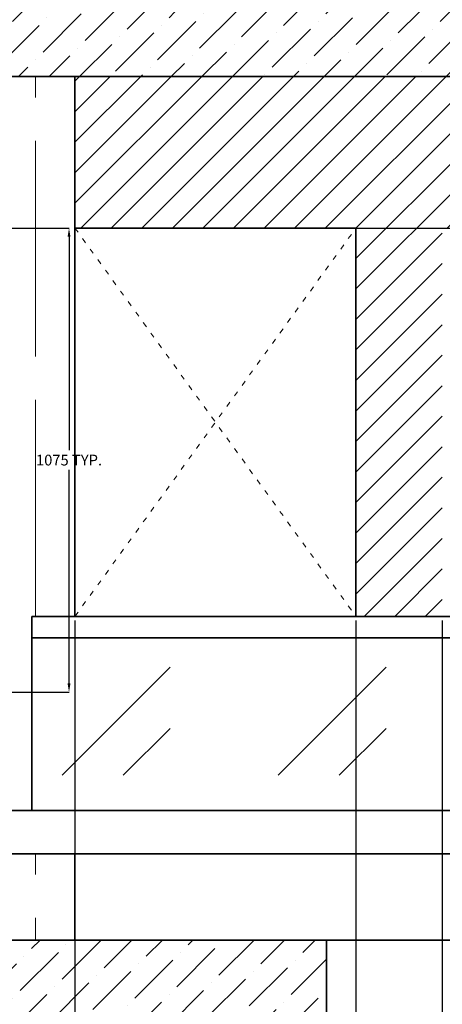
# Model space of a CAD drawing. Units: millimetres. Extents: x -692 to 9639, y -141 to 10345.
# Tile 5 of 19: x 5064 to 6042, y 2699 to 4981. Entities that reach past the tile are written whole.
import ezdxf

# ---------------------------------------------------------------- set-up
doc = ezdxf.new("R2010")
doc.units = ezdxf.units.MM
doc.header["$MEASUREMENT"] = 0
doc.linetypes.add('ACAD_ISO03W100', pattern=[30, 12, -18])
for name, color, linetype, lineweight in [('A-ANNO-DIMS', 2, 'Continuous', 18), ('A-DOOR-SWNG', 3, 'ACAD_ISO03W100', 18), ('A-ELEV', 7, 'Continuous', 35), ('A-ELEV-PATT', 8, 'Continuous', 13)]:
    doc.layers.add(name, color=color, linetype=linetype, lineweight=lineweight)
doc.styles.get("Standard").update_dxf_attribs({"font": 'arial.ttf'})
doc.dimstyles.get("Standard").update_dxf_attribs({"dimtxt": 25, "dimasz": 20, "dimexe": 0.18, "dimexo": 10, "dimgap": 10, "dimtad": 0, "dimtih": 1, "dimtoh": 1, "dimdec": 0, "dimzin": 0, "dimdsep": 46, "dimtxsty": 'Standard', "dimcen": 10, "dimadec": 0, "dimazin": 0, "dimtfac": 1, "dimtdec": 0, "dimtofl": 0, "dimtmove": 0, "dimatfit": 3, "dimfxl": 1, "dimtolj": 1, "dimtzin": 0, "dimarcsym": 0})

# ---------------------------------------------------------------- blocks, each defined once
blk = doc.blocks.new('*D5')
at = {"layer": 'A-ANNO-DIMS', "color": 0, "lineweight": -2, "transparency": 16777216}
for p, q in [((5026.5, 4497.8), (5178, 4497.8)), ((5177.8, 4477.8), (5177.8, 3983)), ((5177.8, 3442.8), (5177.8, 3937.5)), ((5026.5, 3422.8), (5178, 3422.8))]:
    blk.add_line(p, q, dxfattribs=at)
at = {"layer": 'A-ANNO-DIMS', "color": 0, "lineweight": -3, "transparency": 16777216}
for points in [[(5174.5, 4477.8), (5181.1, 4477.8), (5177.8, 4497.8)], [(5174.5, 3442.8), (5181.1, 3442.8), (5177.8, 3422.8)]]:
    blk.add_solid(points, dxfattribs=at)
at = {"layer": 'Defpoints', "color": 0, "lineweight": -3, "transparency": 16777216}
for p in [(5016.5, 4497.8), (5177.8, 4497.8), (5016.5, 3422.8)]:
    blk.add_point(p, dxfattribs=at)
at = {"layer": 'A-ANNO-DIMS', "color": 0, "transparency": 16777216, "insert": (5177.8, 3960.3), "char_height": 25, "attachment_point": 5}
blk.add_mtext('\\A1;1075 TYP.', dxfattribs=at)
blk = doc.blocks.new('*D7')
at = {"layer": 'A-ANNO-DIMS', "color": 0, "lineweight": -2, "transparency": 16777216}
for p, q in [((8481.5, 9848.8), (-649.1, 9848.8)), ((-648.9, 9828.8), (-648.9, 5124.9)), ((-648.9, 375.6), (-648.9, 5079.4)), ((2463.7, 355.6), (-649.1, 355.6))]:
    blk.add_line(p, q, dxfattribs=at)
at = {"layer": 'A-ANNO-DIMS', "color": 0, "lineweight": -3, "transparency": 16777216}
for points in [[(-652.2, 9828.8), (-645.6, 9828.8), (-648.9, 9848.8)], [(-652.2, 375.6), (-645.6, 375.6), (-648.9, 355.6)]]:
    blk.add_solid(points, dxfattribs=at)
at = {"layer": 'Defpoints', "color": 0, "lineweight": -3, "transparency": 16777216}
for p in [(-648.9, 9848.8), (8491.5, 9848.8), (2473.7, 355.6)]:
    blk.add_point(p, dxfattribs=at)
at = {"layer": 'A-ANNO-DIMS', "color": 0, "transparency": 16777216, "insert": (-648.9, 5102.2), "char_height": 25, "attachment_point": 5}
blk.add_mtext('\\A1;9493', dxfattribs=at)
blk = doc.blocks.new('*D39')
at = {"layer": 'A-ANNO-DIMS', "color": 0, "lineweight": -2, "transparency": 16777216}
for p, q in [((5191.5, 3588.3), (5191.5, -124.6)), ((5041.5, 3038.3), (5041.5, -124.6)), ((5061.5, -124.4), (5080.1, -124.4)), ((5171.5, -124.4), (5152.9, -124.4))]:
    blk.add_line(p, q, dxfattribs=at)
at = {"layer": 'A-ANNO-DIMS', "color": 0, "lineweight": -3, "transparency": 16777216}
for points in [[(5061.5, -121.1), (5061.5, -127.8), (5041.5, -124.4)], [(5171.5, -121.1), (5171.5, -127.8), (5191.5, -124.4)]]:
    blk.add_solid(points, dxfattribs=at)
at = {"layer": 'Defpoints', "color": 0, "lineweight": -3, "transparency": 16777216}
for p in [(5191.5, 3598.3), (5041.5, 3048.3), (5191.5, -124.4)]:
    blk.add_point(p, dxfattribs=at)
at = {"layer": 'A-ANNO-DIMS', "color": 0, "transparency": 16777216, "insert": (5116.5, -124.4), "char_height": 25, "attachment_point": 5}
blk.add_mtext('\\A1;150', dxfattribs=at)
blk = doc.blocks.new('*D40')
at = {"layer": 'A-ANNO-DIMS', "color": 0, "lineweight": -2, "transparency": 16777216}
for p, q in [((5191.5, 3588.3), (5191.5, -124.6)), ((5841.7, 3588.3), (5841.7, -124.6)), ((5211.5, -124.4), (5464.5, -124.4)), ((5821.7, -124.4), (5568.8, -124.4))]:
    blk.add_line(p, q, dxfattribs=at)
at = {"layer": 'A-ANNO-DIMS', "color": 0, "lineweight": -3, "transparency": 16777216}
for points in [[(5211.5, -121.1), (5211.5, -127.8), (5191.5, -124.4)], [(5821.7, -121.1), (5821.7, -127.8), (5841.7, -124.4)]]:
    blk.add_solid(points, dxfattribs=at)
at = {"layer": 'Defpoints', "color": 0, "lineweight": -3, "transparency": 16777216}
for p in [(5191.5, 3598.3), (5841.7, 3598.3), (5841.7, -124.4)]:
    blk.add_point(p, dxfattribs=at)
at = {"layer": 'A-ANNO-DIMS', "color": 0, "transparency": 16777216, "insert": (5516.6, -124.4), "char_height": 25, "attachment_point": 5}
blk.add_mtext('\\A1;650.2', dxfattribs=at)
blk = doc.blocks.new('*D41')
at = {"layer": 'A-ANNO-DIMS', "color": 0, "lineweight": -2, "transparency": 16777216}
for p, q in [((5841.7, 3588.3), (5841.7, -124.6)), ((6041.7, 3588.3), (6041.7, -124.6)), ((5861.7, -124.4), (5904, -124.4)), ((6021.7, -124.4), (5979.5, -124.4))]:
    blk.add_line(p, q, dxfattribs=at)
at = {"layer": 'A-ANNO-DIMS', "color": 0, "lineweight": -3, "transparency": 16777216}
for points in [[(5861.7, -121.1), (5861.7, -127.8), (5841.7, -124.4)], [(6021.7, -121.1), (6021.7, -127.8), (6041.7, -124.4)]]:
    blk.add_solid(points, dxfattribs=at)
at = {"layer": 'Defpoints', "color": 0, "lineweight": -3, "transparency": 16777216}
for p in [(5841.7, 3598.3), (6041.7, 3598.3), (6041.7, -124.4)]:
    blk.add_point(p, dxfattribs=at)
at = {"layer": 'A-ANNO-DIMS', "color": 0, "transparency": 16777216, "insert": (5941.7, -124.4), "char_height": 25, "attachment_point": 5}
blk.add_mtext('\\A1;200', dxfattribs=at)
blk = doc.blocks.new('*D42')
at = {"layer": 'A-ANNO-DIMS', "color": 0, "lineweight": -2, "transparency": 16777216}
for p, q in [((6041.7, 3588.3), (6041.7, -124.6)), ((6691.7, 3588.3), (6691.7, -124.6)), ((6061.7, -124.4), (6329.1, -124.4)), ((6671.7, -124.4), (6404.4, -124.4))]:
    blk.add_line(p, q, dxfattribs=at)
at = {"layer": 'A-ANNO-DIMS', "color": 0, "lineweight": -3, "transparency": 16777216}
for points in [[(6061.7, -121.1), (6061.7, -127.8), (6041.7, -124.4)], [(6671.7, -121.1), (6671.7, -127.8), (6691.7, -124.4)]]:
    blk.add_solid(points, dxfattribs=at)
at = {"layer": 'Defpoints', "color": 0, "lineweight": -3, "transparency": 16777216}
for p in [(6041.7, 3598.3), (6691.7, 3598.3), (6691.7, -124.4)]:
    blk.add_point(p, dxfattribs=at)
at = {"layer": 'A-ANNO-DIMS', "color": 0, "transparency": 16777216, "insert": (6366.7, -124.4), "char_height": 25, "attachment_point": 5}
blk.add_mtext('\\A1;650', dxfattribs=at)
blk = doc.blocks.new('*D71')
at = {"layer": 'A-ANNO-DIMS', "color": 0, "lineweight": -2, "transparency": 16777216}
for p, q in [((5201.5, 3598.3), (9553.9, 3598.3)), ((9553.7, 3578.3), (9553.7, 3396)), ((9553.7, 3168.3), (9553.7, 3350.5)), ((5101.5, 3148.3), (9553.9, 3148.3))]:
    blk.add_line(p, q, dxfattribs=at)
at = {"layer": 'A-ANNO-DIMS', "color": 0, "lineweight": -3, "transparency": 16777216}
for points in [[(9550.4, 3578.3), (9557.1, 3578.3), (9553.7, 3598.3)], [(9550.4, 3168.3), (9557.1, 3168.3), (9553.7, 3148.3)]]:
    blk.add_solid(points, dxfattribs=at)
at = {"layer": 'Defpoints', "color": 0, "lineweight": -3, "transparency": 16777216}
for p in [(5191.5, 3598.3), (9553.7, 3598.3), (5091.5, 3148.3)]:
    blk.add_point(p, dxfattribs=at)
at = {"layer": 'A-ANNO-DIMS', "color": 0, "transparency": 16777216, "insert": (9553.7, 3373.3), "char_height": 25, "attachment_point": 5}
blk.add_mtext('\\A1;450', dxfattribs=at)
blk = doc.blocks.new('*D72')
at = {"layer": 'A-ANNO-DIMS', "color": 0, "lineweight": -2, "transparency": 16777216}
for p, q in [((5201.5, 4497.8), (9553.9, 4497.8)), ((9553.7, 4477.8), (9553.7, 4070.8)), ((9553.7, 3618.3), (9553.7, 4025.3)), ((5201.5, 3598.3), (9553.9, 3598.3))]:
    blk.add_line(p, q, dxfattribs=at)
at = {"layer": 'A-ANNO-DIMS', "color": 0, "lineweight": -3, "transparency": 16777216}
for points in [[(9550.4, 4477.8), (9557.1, 4477.8), (9553.7, 4497.8)], [(9550.4, 3618.3), (9557.1, 3618.3), (9553.7, 3598.3)]]:
    blk.add_solid(points, dxfattribs=at)
at = {"layer": 'Defpoints', "color": 0, "lineweight": -3, "transparency": 16777216}
for p in [(5191.5, 4497.8), (9553.7, 4497.8), (5191.5, 3598.3)]:
    blk.add_point(p, dxfattribs=at)
at = {"layer": 'A-ANNO-DIMS', "color": 0, "transparency": 16777216, "insert": (9553.7, 4048), "char_height": 25, "attachment_point": 5}
blk.add_mtext('\\A1;899.5', dxfattribs=at)
blk = doc.blocks.new('*D73')
at = {"layer": 'A-ANNO-DIMS', "color": 0, "lineweight": -2, "transparency": 16777216}
for p, q in [((8301.5, 4698.8), (9553.9, 4698.8)), ((9553.7, 4678.8), (9553.7, 4621)), ((9553.7, 4517.8), (9553.7, 4575.5)), ((5201.5, 4497.8), (9553.9, 4497.8))]:
    blk.add_line(p, q, dxfattribs=at)
at = {"layer": 'A-ANNO-DIMS', "color": 0, "lineweight": -3, "transparency": 16777216}
for points in [[(9550.4, 4678.8), (9557.1, 4678.8), (9553.7, 4698.8)], [(9550.4, 4517.8), (9557.1, 4517.8), (9553.7, 4497.8)]]:
    blk.add_solid(points, dxfattribs=at)
at = {"layer": 'Defpoints', "color": 0, "lineweight": -3, "transparency": 16777216}
for p in [(8291.5, 4698.8), (9553.7, 4698.8), (5191.5, 4497.8)]:
    blk.add_point(p, dxfattribs=at)
at = {"layer": 'A-ANNO-DIMS', "color": 0, "transparency": 16777216, "insert": (9553.7, 4598.3), "char_height": 25, "attachment_point": 5}
blk.add_mtext('\\A1;201', dxfattribs=at)

msp = doc.modelspace()

# ---------------------------------------------------------------- hatches: boundary and pattern name
at = {"layer": 'A-ELEV-PATT'}
h = msp.add_hatch(dxfattribs=at)
h.set_pattern_fill('GOST_WOOD', color=256, scale=50)
h.set_pattern_definition([(90, (0, 0), (300, -2e-14), [500, -100]), (90, (100, -100), (300, -2e-14), [300, -75, 150, -75]), (90, (200, -250), (300, -2e-14), [500, -100])])
edge = h.paths.add_edge_path()
edge.add_line((5191.547, 8748.772), (3791.547, 8748.772))
edge.add_line((3791.547, 8748.772), (3791.547, 8848.772))
edge.add_line((3791.547, 8848.772), (5191.547, 8848.772))
edge.add_line((5191.547, 8848.772), (5191.547, 9348.772))
edge.add_line((5191.547, 9348.772), (4755.992, 9348.772))
edge.add_line((4755.992, 9348.772), (4755.854, 9348.465))
edge.add_line((4755.854, 9348.465), (4755.734, 9348.772))
edge.add_line((4755.734, 9348.772), (4053.129, 9348.772))
edge.add_line((4053.129, 9348.772), (4052.99, 9348.465))
edge.add_line((4052.99, 9348.465), (4052.871, 9348.772))
edge.add_line((4052.871, 9348.772), (3701.731, 9348.772))
edge.add_line((3701.731, 9348.772), (3701.593, 9348.465))
edge.add_line((3701.593, 9348.465), (3701.474, 9348.772))
edge.add_line((3701.474, 9348.772), (3368.199, 9348.772))
edge.add_line((3368.199, 9348.772), (3368.061, 9348.465))
edge.add_line((3368.061, 9348.465), (3367.942, 9348.772))
edge.add_line((3367.942, 9348.772), (3191.547, 9348.772))
edge.add_line((3191.547, 9348.772), (3191.547, 3210.058))
edge.add_spline(control_points=[(3191.547, 3210.058), (3198.467, 3207.5), (3283.859, 3166.656), (3324.053, 2995.08), (3234.02, 2920.058), (3220.783, 2911.684)], knot_values=[13649.89756952, 13649.89756952, 13649.89756952, 13649.89756952, 13672.14990348, 13935.42377748, 13974.4426778, 13974.4426778, 13974.4426778, 13974.4426778], degree=3, periodic=0)
edge.add_spline(control_points=[(3220.783, 2911.684), (3225.148, 2890.107), (3226.864, 2868.931), (3226.144, 2848.27)], knot_values=[8828.69997321, 8828.69997321, 8828.69997321, 8828.69997321, 8890.6429847, 8890.6429847, 8890.6429847, 8890.6429847], degree=3, periodic=0)
edge.add_line((3226.144, 2848.27), (5191.547, 2848.27))
edge.add_line((5191.547, 2848.27), (5191.547, 3048.27))
edge.add_line((5191.547, 3048.27), (5041.547, 3048.27))
edge.add_line((5041.547, 3048.27), (5041.547, 3148.27))
edge.add_line((5041.547, 3148.27), (5091.547, 3148.27))
edge.add_line((5091.547, 3148.27), (5091.547, 3598.27))
edge.add_line((5091.547, 3598.27), (5191.547, 3598.27))
edge.add_line((5191.547, 3598.27), (5191.547, 4848.772))
edge.add_line((5191.547, 4848.772), (3791.547, 4848.772))
edge.add_line((3791.547, 4848.772), (3791.547, 6848.772))
edge.add_line((3791.547, 6848.772), (5091.547, 6848.772))
edge.add_line((5091.547, 6848.772), (5091.547, 7298.772))
edge.add_line((5091.547, 7298.772), (5191.547, 7298.772))
edge.add_line((5191.547, 7298.772), (5191.547, 8748.772))
h.paths.add_polyline_path([(5016.547, 8198.772), (5016.547, 7123.772), (3941.547, 7123.772), (3941.547, 8198.772)], flags=16)
h.paths.add_polyline_path([(4941.547, 8123.772), (4941.547, 7198.772), (4016.547, 7198.772), (4016.547, 8123.772)], flags=0)
h.paths.add_polyline_path([(4616.547, 8073.772), (4616.547, 7248.772), (4341.547, 7248.772), (4341.547, 8073.772)], flags=0)
h.paths.add_polyline_path([(4641.547, 8073.772), (4891.547, 8073.772), (4891.547, 7248.772), (4641.547, 7248.772)], flags=0)
h.paths.add_polyline_path([(4666.547, 8048.772), (4866.547, 8048.772), (4866.547, 7273.772), (4666.547, 7273.772)], flags=0)
h.paths.add_polyline_path([(4316.547, 8073.772), (4316.547, 7248.772), (4066.547, 7248.772), (4066.547, 8073.772)], flags=0)
h.paths.add_polyline_path([(4291.547, 8048.772), (4291.547, 7273.772), (4091.547, 7273.772), (4091.547, 8048.772)], flags=0)
h.paths.add_polyline_path([(5016.547, 4497.772), (5016.547, 3422.772), (3941.547, 3422.772), (3941.547, 4497.772)], flags=16)
h.paths.add_polyline_path([(4941.547, 4422.772), (4941.547, 3497.772), (4016.547, 3497.772), (4016.547, 4422.772)], flags=0)
h.paths.add_polyline_path([(4616.547, 4372.772), (4616.547, 3547.772), (4341.547, 3547.772), (4341.547, 4372.772)], flags=0)
h.paths.add_polyline_path([(4641.547, 4372.772), (4891.547, 4372.772), (4891.547, 3547.772), (4641.547, 3547.772)], flags=0)
h.paths.add_polyline_path([(4316.547, 4372.772), (4316.547, 3547.772), (4066.547, 3547.772), (4066.547, 4372.772)], flags=0)
h.paths.add_polyline_path([(4666.547, 4347.772), (4866.547, 4347.772), (4866.547, 3572.772), (4666.547, 3572.772)], flags=0)
h.paths.add_polyline_path([(4291.547, 4347.772), (4291.547, 3572.772), (4091.547, 3572.772), (4091.547, 4347.772)], flags=0)
h = msp.add_hatch(dxfattribs=at)
h.set_pattern_fill('ANSI31', color=256, scale=400)
h.paths.add_polyline_path([(6891.746, 6698.772), (5191.547, 6698.772), (5191.547, 6348.772), (5841.547, 6348.772), (5841.547, 5448.772), (6041.547, 5448.772), (6041.547, 6348.772), (6691.547, 6348.772), (6691.547, 5448.772), (6891.746, 5448.772)])
h.paths.add_polyline_path([(5191.547, 6698.772), (3941.547, 6698.772), (3941.547, 5448.772), (4006.259, 5448.772), (4006.259, 6423.772), (5081.259, 6423.772), (5081.259, 5448.772), (5191.547, 5448.772), (5191.547, 6348.772)])
h.paths.add_polyline_path([(6891.746, 4848.772), (5191.547, 4848.772), (5191.547, 4497.772), (5841.746, 4497.772), (5841.746, 3598.27), (6041.746, 3598.27), (6041.746, 4497.772), (6691.746, 4497.772), (6691.746, 3598.27), (6891.746, 3598.27)])
h.paths.add_polyline_path([(6891.746, 8748.772), (5191.547, 8748.772), (5191.547, 8198.772), (5841.547, 8198.772), (5841.547, 7298.772), (6041.547, 7298.772), (6041.547, 8198.772), (6691.547, 8198.772), (6691.547, 7298.772), (6891.746, 7298.772)])
h = msp.add_hatch(dxfattribs=at)
h.set_pattern_fill('ANSI36', color=256, scale=400)
h.paths.add_polyline_path([(8691.547, 6848.772), (3791.547, 6848.772), (3791.547, 4848.772), (8691.547, 4848.772), (8691.547, 4998.772), (3941.547, 4998.772), (3941.547, 6698.772), (8691.547, 6698.772)])
h = msp.add_hatch(dxfattribs=at)
h.set_pattern_fill('ANSI36', color=256, scale=400)
edge = h.paths.add_edge_path()
edge.add_line((5773.746, 2848.27), (3226.144, 2848.27))
edge.add_spline(control_points=[(3226.144, 2848.27), (3225.984, 2843.657), (3225.702, 2839.069), (3225.3, 2834.508)], knot_values=[8814.86919927, 8814.86919927, 8814.86919927, 8814.86919927, 8828.69997321, 8828.69997321, 8828.69997321, 8828.69997321], degree=3, periodic=0)
edge.add_spline(control_points=[(3225.3, 2834.508), (3299.425, 2803.396), (3368.378, 2761.363), (3420.651, 2717.101)], knot_values=[12552.99587302, 12552.99587302, 12552.99587302, 12552.99587302, 12712.02358035, 12712.02358035, 12712.02358035, 12712.02358035], degree=3, periodic=0)
edge.add_spline(control_points=[(3420.651, 2717.101), (3432.322, 2714.914), (3488.975, 2701.706), (3489.525, 2687.271), (3463.702, 2676.006)], knot_values=[10852.53626518, 10852.53626518, 10852.53626518, 10852.53626518, 10887.45464539, 11042.13010686, 11042.13010686, 11042.13010686, 11042.13010686], degree=3, periodic=0)
edge.add_spline(control_points=[(3463.702, 2676.006), (3472.194, 2666.716), (3479.817, 2657.445), (3486.469, 2648.27)], knot_values=[12471.26094935, 12471.26094935, 12471.26094935, 12471.26094935, 12504.23047843, 12504.23047843, 12504.23047843, 12504.23047843], degree=3, periodic=0)
edge.add_line((3486.469, 2648.27), (5373.746, 2648.27))
edge.add_line((5373.746, 2648.27), (5373.746, 855.575))
edge.add_line((5373.746, 855.575), (5773.746, 855.575))
edge.add_line((5773.746, 855.575), (5773.746, 2848.27))

# ---------------------------------------------------------------- linework, layer by layer
at = {"layer": 'A-DOOR-SWNG'}
for p, q in [((5191.547, 3598.27), (5841.746, 4497.772)), ((5191.547, 4497.772), (5841.746, 3598.27))]:
    msp.add_line(p, q, dxfattribs=at)
at = {"layer": 'A-ELEV'}
for p, q in [((3791.547, 4848.772), (8691.547, 4848.772)), ((5191.547, 3598.27), (5191.547, 4848.772)), ((5191.547, 4497.772), (5841.746, 4497.772)), ((5841.746, 3598.27), (5841.746, 4497.772)), ((5191.547, 3598.27), (5091.547, 3598.27)), ((5091.547, 3598.27), (5091.547, 3148.27)), ((5191.547, 3598.27), (7766.547, 3598.27)), ((5091.547, 3548.27), (7766.547, 3548.27)), ((5411.99, 3480.203), (5161.99, 3230.203)), ((5911.99, 3480.203), (5661.99, 3230.203)), ((5411.99, 3338.782), (5303.412, 3230.203)), ((5911.99, 3338.782), (5803.412, 3230.203)), ((5041.547, 3148.27), (5191.547, 3148.27)), ((5191.547, 3148.27), (8491.547, 3148.27)), ((5191.547, 3048.27), (5041.547, 3048.27)), ((5191.547, 2848.27), (5191.547, 3048.27)), ((5191.547, 3048.27), (8491.547, 3048.27)), ((2773.746, 2848.27), (5773.746, 2848.27)), ((5773.746, 2848.27), (5773.746, 855.575)), ((5773.746, 2848.27), (8341.547, 2848.27))]:
    msp.add_line(p, q, dxfattribs=at)

# ---------------------------------------------------------------- dimensions: what is measured, and where the dimension line sits
at = {"layer": 'A-ANNO-DIMS'}
for base, p1, p2, override, picture, middle in [((-648.912, 9848.772), (2473.746, 355.575), (8491.547, 9848.772), {"dimdec": 0, "dimlfac": 1, "dimrnd": 0, "dimzin": 0, "dimdsep": 46, "dimlunit": 2}, '*D7', (-648.912, 5102.173)), ((9553.746, 4698.772), (5191.547, 4497.772), (8291.547, 4698.772), {"dimdec": 0, "dimlfac": 1, "dimrnd": 0, "dimzin": 0, "dimdsep": 46, "dimlunit": 2}, '*D73', (9553.746, 4598.272)), ((9553.746, 4497.772), (5191.547, 3598.27), (5191.547, 4497.772), {"dimdec": 1, "dimlfac": 1, "dimrnd": 0, "dimzin": 0, "dimdsep": 46, "dimlunit": 2}, '*D72', (9553.746, 4048.021)), ((9553.746, 3598.27), (5091.547, 3148.27), (5191.547, 3598.27), {"dimdec": 0, "dimlfac": 1, "dimrnd": 0, "dimzin": 0, "dimdsep": 46, "dimlunit": 2}, '*D71', (9553.746, 3373.27))]:
    dim = msp.add_linear_dim(base=base, p1=p1, p2=p2, angle=90, dimstyle='Standard', override=override, dxfattribs=at)
    dim.commit()
    dim.dimension.update_dxf_attribs({"geometry": picture, "text_midpoint": middle})
dim = msp.add_linear_dim(base=(5177.797, 4497.772), p1=(5016.547, 3422.772), p2=(5016.547, 4497.772), angle=90, text='<> TYP.', dimstyle='Standard', override={"dimdec": 0, "dimrnd": 0, "dimzin": 0, "dimlunit": 2}, dxfattribs=at)
dim.commit()
dim.dimension.update_dxf_attribs({"geometry": '*D5', "text_midpoint": (5177.797, 3960.272)})
for base, p1, p2, override, picture, middle in [((5191.547, -124.425), (5041.547, 3048.27), (5191.547, 3598.27), {"dimdec": 0, "dimlfac": 1, "dimrnd": 0, "dimzin": 0, "dimdsep": 46, "dimlunit": 2}, '*D39', (5116.547, -124.425)), ((5841.746, -124.425), (5191.547, 3598.27), (5841.746, 3598.27), {"dimdec": 1, "dimlfac": 1, "dimrnd": 0, "dimzin": 0, "dimdsep": 46, "dimlunit": 2}, '*D40', (5516.646, -124.425)), ((6041.746, -124.425), (5841.746, 3598.27), (6041.746, 3598.27), {"dimdec": 0, "dimlfac": 1, "dimrnd": 0, "dimzin": 0, "dimdsep": 46, "dimlunit": 2}, '*D41', (5941.746, -124.425)), ((6691.746, -124.425), (6041.746, 3598.27), (6691.746, 3598.27), {"dimdec": 0, "dimlfac": 1, "dimrnd": 0, "dimzin": 0, "dimdsep": 46, "dimlunit": 2}, '*D42', (6366.746, -124.425))]:
    dim = msp.add_linear_dim(base=base, p1=p1, p2=p2, dimstyle='Standard', override=override, dxfattribs=at)
    dim.commit()
    dim.dimension.update_dxf_attribs({"geometry": picture, "text_midpoint": middle})

doc.saveas('drawing.dxf')
